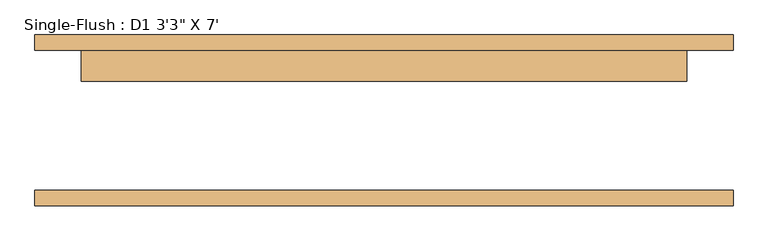
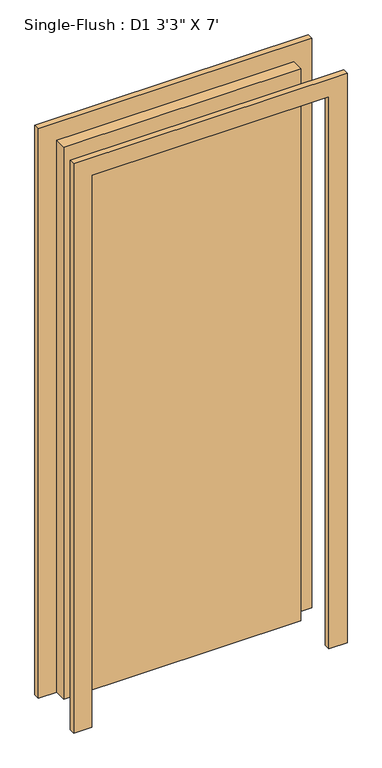
"""IFC4 building model written with IfcOpenShell, lengths in millimetres: door geometry."""

from ifc_helpers import new_model, si_unit, frame, origin, origin_with_axes, place, context, project, spatial, polyline, outline, extrude, source, transform, mapped, element, save


def door_02e7543a(model_context):
    return source(origin(), model_context, "Body", "SweptSolid", [
        extrude(outline(polyline([(2514.6, -571.5), (0.0, -571.5), (0.0, -495.3), (2438.4, -495.3), (2438.4, 495.3), (0.0, 495.3), (0.0, 571.5), (2514.6, 571.5), (2514.6, -571.5)])), frame((0.0, 114.3, 0.0), z_axis=(0.0, 1.0, 0.0), x_axis=(0.0, 0.0, 1.0)), (0.0, 0.0, 1.0), 25.4),
        extrude(outline(polyline([(2514.6, 571.5), (2514.6, -571.5), (0.0, -571.5), (0.0, -495.3), (2438.4, -495.3), (2438.4, 495.3), (0.0, 495.3), (0.0, 571.5), (2514.6, 571.5)])), frame((0.0, -139.7, 0.0), z_axis=(0.0, 1.0, 0.0), x_axis=(0.0, 0.0, 1.0)), (0.0, 0.0, 1.0), 25.4),
        extrude(outline(polyline([(495.3, 63.5), (-495.3, 63.5), (-495.3, 114.3), (495.3, 114.3), (495.3, 63.5)])), origin_with_axes(), (0.0, 0.0, 1.0), 2438.4),
    ])


if __name__ == "__main__":
    model = new_model("IFC4")
    model_context = context("Model", 3, world=origin())
    ifc_project = project(units=[si_unit("LENGTHUNIT", "METRE", prefix="MILLI")], contexts=[model_context])
    site = spatial("IfcSite", under=ifc_project)
    building = spatial("IfcBuilding", under=site)
    placement = place(None, origin())
    door_shape = door_02e7543a(model_context)
    element("IfcDoor", 1, ObjectType="Single-Flush : D1 3'3\" X 7'", at=placement, inside=building, context=model_context, shape_type="MappedRepresentation", body=[
        mapped(door_shape, transform((0.0, 0.0, 0.0), x_axis=(1.0, 0.0, 0.0), y_axis=(0.0, 1.0, 0.0), z_axis=(0.0, 0.0, 1.0))),
    ])
    save(model, "model.ifc")

# Revit data of these elements
# Type "Single-Flush : D1 3'3\" X 7'"
#   Type Mark = "9"
#   Construction Type Id = "MDOOR"
#   Assembly Code = "C1020"
#   Analytic Construction = "Metal"
#   Thickness = 0' - 2"
#   Heat Transfer Coefficient (U) = 0.651978 BTU/(h·ft²·°F)
#   Height = 8' - 0"
#   Trim Projection Ext = 0' - 1"
#   Trim Projection Int = 0' - 1"
#   Trim Width = 0' - 3"
#   Width = 3' - 3"
#   Define Thermal Properties by = 1
#   Door Material = Door - Panel
#   Frame Material = Door - Frame
#   Visual Light Transmittance = 0
#   Solar Heat Gain Coefficient = 0
#   Function = (empty or 0)
#   Wall Closure = (empty or 0)
# Element 1 (IfcDoor, "Single-Flush : D1 3'3\" X 7'")
#   Materials on its faces: "Door - Frame", "Door - Panel"
# Materials
#   "Door - Panel": class "Wood", colour RGB 210 159 95, transparency 0, Cost = 0
#   "Door - Frame": colour RGB 118 70 51, transparency 0, Cost = 0
